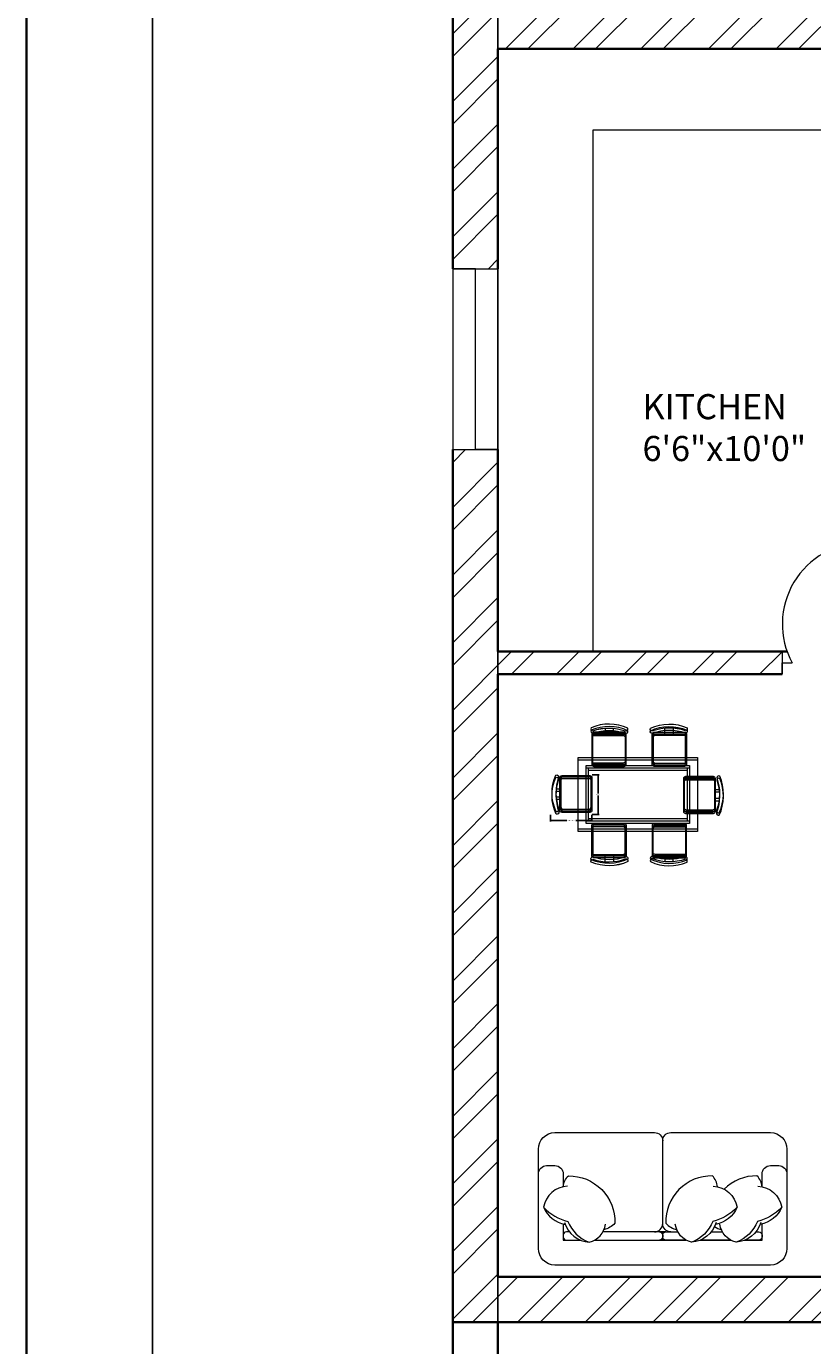
# Model space of a CAD drawing. Units: inches. Extents: x 2552 to 3217, y 1417 to 2737.
# Tile 2 of 25: x 2552 to 2709, y 1622 to 1885. Entities that reach past the tile are written whole.
import ezdxf

# ---------------------------------------------------------------- set-up
doc = ezdxf.new("R2010")
doc.units = ezdxf.units.IN
for name, color, linetype, lineweight in [('A-ANNO-DIMS', 2, 'Continuous', 18), ('A-ANNO-TTLB', 7, 'Continuous', 35), ('A-AREA-IDEN', 7, 'Continuous', 18), ('A-DOOR', 21, 'Continuous', 18), ('A-FLOR-CASE', 9, 'Continuous', 18), ('A-FURN', 8, 'Continuous', 13), ('A-GLAZ', 161, 'Continuous', 18), ('A-WALL', 7, 'Continuous', 35), ('A-WALL-PATT', 217, 'Continuous', 13)]:
    doc.layers.add(name, color=color, linetype=linetype, lineweight=lineweight)
doc.styles.get("Standard").update_dxf_attribs({"font": 'arial.ttf'})
doc.dimstyles.get("Standard").update_dxf_attribs({"dimtxt": 0.18, "dimasz": 0.18, "dimexe": 0.18, "dimexo": 0.0625, "dimgap": 0.09, "dimtad": 0, "dimtih": 1, "dimtoh": 1, "dimdec": 4, "dimzin": 0, "dimdsep": 46, "dimtxsty": 'Standard', "dimcen": 0.09, "dimadec": 0, "dimazin": 0, "dimtfac": 1, "dimtdec": 4, "dimtofl": 0, "dimtmove": 0, "dimatfit": 3, "dimfxl": 1, "dimtolj": 1, "dimtzin": 0, "dimarcsym": 0})

# ---------------------------------------------------------------- blocks, each defined once
blk = doc.blocks.new('TABLE-DINING-RECT')
for points in [[(0, 14.74), (23.77, 14.74), (23.77, 0.48), (0, 0.48)], [(0, 14.74), (23.77, 14.74), (23.77, 0.48), (0, 0.48)], [(0, 14.26), (23.77, 14.26), (23.77, 0), (0, 0)], [(0, 14.26), (23.77, 14.26), (23.77, 0), (0, 0)], [(1.58, 13.15), (22.19, 13.15), (22.19, 2.06), (1.58, 2.06)], [(1.58, 13.15), (22.19, 13.15), (22.19, 2.06), (1.58, 2.06)], [(1.58, 12.68), (22.19, 12.68), (22.19, 1.59), (1.58, 1.59)], [(1.58, 12.68), (22.19, 12.68), (22.19, 1.58), (1.58, 1.58)], [(2.06, 12.68), (21.71, 12.68), (21.71, 2.54), (2.06, 2.54)], [(2.06, 12.68), (21.71, 12.68), (21.71, 2.54), (2.06, 2.54)], [(2.06, 12.2), (21.71, 12.2), (21.71, 2.06), (2.06, 2.06)], [(2.06, 12.2), (21.71, 12.2), (21.71, 2.06), (2.06, 2.06)]]:
    blk.add_lwpolyline(points, close=True)
blk = doc.blocks.new('DINING-CHAIR-WEST')
for points in [[(1.37, 0.99, -0.578392), (0.83, 0.5, -0.214524), (0.73, 7.8, -0.552014), (1.32, 7.46, 0.175809), (1.37, 0.99)], [(1.37, 0.99, -0.578392), (0.83, 0.49, -0.214524), (0.73, 7.8, -0.552014), (1.32, 7.46, 0.175809), (1.37, 0.99)], [(1.37, 0.51, -0.578392), (0.83, 0.02, -0.214524), (0.73, 7.33, -0.552014), (1.32, 6.98, 0.175809), (1.37, 0.51)], [(1.37, 0.51, -0.578392), (0.83, 0.02, -0.214524), (0.73, 7.33, -0.552014), (1.32, 6.98, 0.175809), (1.37, 0.51)], [(1.58, 7.27, -0.414214), (2, 7.69), (7.53, 7.69, -0.414214), (7.95, 7.27), (7.95, 1.26, -0.414214), (7.53, 0.84), (2, 0.84, -0.414214), (1.58, 1.26), (1.58, 7.27)], [(1.58, 7.27, -0.414214), (2, 7.69), (7.53, 7.69, -0.414214), (7.95, 7.27), (7.95, 1.26, -0.414214), (7.53, 0.84), (2, 0.84, -0.414214), (1.58, 1.26), (1.58, 7.27)], [(1.58, 6.8, -0.414214), (2, 7.22), (7.53, 7.22, -0.414214), (7.95, 6.8), (7.95, 0.78, -0.414214), (7.53, 0.36), (2, 0.36, -0.414214), (1.58, 0.78), (1.58, 6.8)], [(1.58, 6.8, -0.414214), (2, 7.22), (7.53, 7.22, -0.414214), (7.95, 6.8), (7.95, 0.78, -0.414214), (7.53, 0.36), (2, 0.36, -0.414214), (1.58, 0.78), (1.58, 6.8)], [(1.58, 3.37), (0.82, 3.37, 0.064759)], [(1.58, 3.37), (0.82, 3.37, 0.064759)], [(1.58, 2.9), (0.82, 2.9, 0.064759)], [(1.58, 2.9), (0.82, 2.9, 0.064759)]]:
    blk.add_lwpolyline(points, format="xyb")
for points in [[(1.77, 7.27), (1.77, 1.45, 0.414214), (2.19, 1.03), (7.34, 1.03, 0.414214), (7.76, 1.45), (7.76, 7.27, 0.512069), (7.34, 7.5), (2.19, 7.5, 0.512069)], [(1.77, 7.27), (1.77, 1.45, 0.414214), (2.19, 1.03), (7.34, 1.03, 0.414214), (7.76, 1.45), (7.76, 7.27, 0.512069), (7.34, 7.5), (2.19, 7.5, 0.512069)], [(1.77, 6.79), (1.77, 0.97, 0.414214), (2.19, 0.55), (7.34, 0.55, 0.414214), (7.76, 0.97), (7.76, 6.79, 0.512069), (7.34, 7.03), (2.19, 7.03, 0.512069)], [(1.77, 6.79), (1.77, 0.97, 0.414214), (2.19, 0.55), (7.34, 0.55, 0.414214), (7.76, 0.97), (7.76, 6.79, 0.512069), (7.34, 7.03), (2.19, 7.03, 0.512069)]]:
    blk.add_lwpolyline(points, format="xyb", close=True)
for points in [[(0.81, 5.05), (1.58, 5.05)], [(0.81, 5.05), (1.58, 5.05)], [(0.81, 4.58), (1.58, 4.58)], [(0.81, 4.58), (1.58, 4.58)]]:
    blk.add_lwpolyline(points)
blk = doc.blocks.new('DINING-CHAIR-EAST')
for points in [[(6.37, 7.27, 0.414214), (5.95, 7.69), (0.42, 7.69, 0.414214), (0, 7.27), (0, 1.26, 0.414214), (0.42, 0.84), (5.95, 0.84, 0.414214), (6.37, 1.26), (6.37, 7.27)], [(6.37, 7.27, 0.414214), (5.95, 7.69), (0.42, 7.69, 0.414214), (0, 7.27), (0, 1.26, 0.414214), (0.42, 0.84), (5.95, 0.84, 0.414214), (6.37, 1.26), (6.37, 7.27)], [(6.37, 6.8, 0.414214), (5.95, 7.22), (0.42, 7.22, 0.414214), (0, 6.8), (0, 0.78, 0.414214), (0.42, 0.36), (5.95, 0.36, 0.414214), (6.37, 0.78), (6.37, 6.8)], [(6.37, 6.8, 0.414214), (5.95, 7.22), (0.42, 7.22, 0.414214), (0, 6.8), (0, 0.78, 0.414214), (0.42, 0.36), (5.95, 0.36, 0.414214), (6.37, 0.78), (6.37, 6.8)], [(6.63, 7.46, -0.175809), (6.58, 0.99, 0.578392), (7.12, 0.5, 0.214524), (7.22, 7.8, 0.552014), (6.63, 7.46, -0.065079)], [(6.63, 7.46, -0.175809), (6.58, 0.99, 0.578392), (7.12, 0.49, 0.214524), (7.22, 7.8, 0.552014), (6.63, 7.46, -0.065079)], [(6.63, 6.98, -0.175809), (6.58, 0.51, 0.578392), (7.12, 0.02, 0.214524), (7.22, 7.33, 0.552014), (6.63, 6.98, -0.065079)], [(6.63, 6.98, -0.175809), (6.58, 0.51, 0.578392), (7.12, 0.02, 0.214524), (7.22, 7.33, 0.552014), (6.63, 6.98, -0.065079)], [(6.37, 3.37), (7.13, 3.37, -0.064759)], [(6.37, 3.37), (7.13, 3.37, -0.064759)], [(6.37, 2.9), (7.13, 2.9, -0.064759)], [(6.37, 2.9), (7.13, 2.9, -0.064759)]]:
    blk.add_lwpolyline(points, format="xyb")
for points in [[(6.18, 7.27), (6.18, 1.45, -0.414214), (5.76, 1.03), (0.61, 1.03, -0.414214), (0.19, 1.45), (0.19, 7.27, -0.512069), (0.61, 7.5), (5.76, 7.5, -0.512069)], [(6.18, 7.27), (6.18, 1.45, -0.414214), (5.76, 1.03), (0.61, 1.03, -0.414214), (0.19, 1.45), (0.19, 7.27, -0.512069), (0.61, 7.5), (5.76, 7.5, -0.512069)], [(6.18, 6.79), (6.18, 0.97, -0.414214), (5.76, 0.55), (0.61, 0.55, -0.414214), (0.19, 0.97), (0.19, 6.79, -0.512069), (0.61, 7.03), (5.76, 7.03, -0.512069)], [(6.18, 6.79), (6.18, 0.97, -0.414214), (5.76, 0.55), (0.61, 0.55, -0.414214), (0.19, 0.97), (0.19, 6.79, -0.512069), (0.61, 7.03), (5.76, 7.03, -0.512069)]]:
    blk.add_lwpolyline(points, format="xyb", close=True)
for points in [[(7.14, 5.05), (6.37, 5.05)], [(7.14, 5.05), (6.37, 5.05)], [(7.14, 4.58), (6.37, 4.58)], [(7.14, 4.58), (6.37, 4.58)]]:
    blk.add_lwpolyline(points)
blk = doc.blocks.new('DINING-CHAIR-SOUTH-EAST')
for points in [[(6.8, 2.06, 0.414214), (7.22, 2.48), (7.22, 8.01, 0.414214), (6.8, 8.43), (0.78, 8.43, 0.414214), (0.36, 8.01), (0.36, 2.48, 0.414214), (0.78, 2.06), (6.8, 2.06)], [(6.8, 2.06, 0.414214), (7.22, 2.48), (7.22, 8.01, 0.414214), (6.8, 8.43), (0.78, 8.43, 0.414214), (0.36, 8.01), (0.36, 2.48, 0.414214), (0.78, 2.06), (6.8, 2.06)], [(6.8, 1.58, 0.414214), (7.22, 2), (7.22, 7.53, 0.414214), (6.8, 7.95), (0.78, 7.95, 0.414214), (0.36, 7.53), (0.36, 2, 0.414214), (0.78, 1.58), (6.8, 1.58)], [(6.8, 1.58, 0.414214), (7.22, 2), (7.22, 7.53, 0.414214), (6.8, 7.95), (0.78, 7.95, 0.414214), (0.36, 7.53), (0.36, 2, 0.414214), (0.78, 1.58), (6.8, 1.58)], [(6.98, 1.8, -0.175809), (0.51, 1.85, 0.578392), (0.02, 1.31, 0.214524), (7.33, 1.21, 0.552014), (6.98, 1.8, -0.065079)], [(6.98, 1.8, -0.175809), (0.51, 1.85, 0.578392), (0.02, 1.31, 0.214524), (7.33, 1.21, 0.552014), (6.98, 1.8, -0.065079)], [(6.98, 1.32, -0.175809), (0.51, 1.37, 0.578392), (0.02, 0.83, 0.214524), (7.33, 0.74, 0.552014), (6.98, 1.32, -0.065079)], [(6.98, 1.32, -0.175809), (0.51, 1.37, 0.578392), (0.02, 0.83, 0.214524), (7.33, 0.74, 0.552014), (6.98, 1.32, -0.065079)], [(2.9, 2.06), (2.9, 1.3, -0.064759)], [(2.9, 2.06), (2.9, 1.3, -0.064759)], [(2.9, 1.58), (2.9, 0.82, -0.064759)], [(2.9, 1.58), (2.9, 0.82, -0.064759)]]:
    blk.add_lwpolyline(points, format="xyb")
for points in [[(6.79, 2.25), (0.97, 2.25, -0.414214), (0.55, 2.67), (0.55, 7.82, -0.414214), (0.97, 8.24), (6.79, 8.24, -0.512069), (7.03, 7.82), (7.03, 2.67, -0.512069)], [(6.79, 2.25), (0.97, 2.25, -0.414214), (0.55, 2.67), (0.55, 7.82, -0.414214), (0.97, 8.24), (6.79, 8.24, -0.512069), (7.03, 7.82), (7.03, 2.67, -0.512069)], [(6.79, 1.77), (0.97, 1.77, -0.414214), (0.55, 2.19), (0.55, 7.34, -0.414214), (0.97, 7.76), (6.79, 7.76, -0.512069), (7.03, 7.34), (7.03, 2.19, -0.512069)], [(6.79, 1.77), (0.97, 1.77, -0.414214), (0.55, 2.19), (0.55, 7.34, -0.414214), (0.97, 7.76), (6.79, 7.76, -0.512069), (7.03, 7.34), (7.03, 2.19, -0.512069)]]:
    blk.add_lwpolyline(points, format="xyb", close=True)
for points in [[(4.58, 1.28), (4.58, 2.06)], [(4.58, 1.28), (4.58, 2.06)], [(4.58, 0.81), (4.58, 1.58)], [(4.58, 0.81), (4.58, 1.58)]]:
    blk.add_lwpolyline(points)
blk = doc.blocks.new('WIN-36')
for p, q in [((4.5, 36), (0, 36)), ((0, 36), (9, 36)), ((0, 36), (0, 0)), ((4.5, 0), (4.5, 36)), ((9, 36), (9, 0)), ((0, 0), (9, 0)), ((9, 0), (4.5, 0))]:
    blk.add_line(p, q)
blk = doc.blocks.new('*D37')
at = {"layer": 'A-ANNO-DIMS', "color": 0, "lineweight": -2, "transparency": 16777216}
for p, q in [((2656.84, 1727.55), (2656.84, 1726.2)), ((2657.02, 1726.38), (2660.07, 1726.38)), ((2664.89, 1726.38), (2661.83, 1726.38)), ((2665.07, 1727.55), (2665.07, 1726.2))]:
    blk.add_line(p, q, dxfattribs=at)
at = {"layer": 'A-ANNO-DIMS', "color": 0, "transparency": 16777216}
for points in [[(2657.02, 1726.41), (2657.02, 1726.35), (2656.84, 1726.38)], [(2664.89, 1726.41), (2664.89, 1726.35), (2665.07, 1726.38)]]:
    blk.add_solid(points, dxfattribs=at)
at = {"layer": 'Defpoints', "color": 0, "transparency": 16777216}
for p in [(2656.84, 1727.62), (2665.07, 1727.62), (2665.07, 1726.38)]:
    blk.add_point(p, dxfattribs=at)
at = {"layer": 'A-ANNO-DIMS', "color": 0, "transparency": 16777216, "insert": (2660.95, 1726.38), "char_height": 0.18, "attachment_point": 5}
blk.add_mtext('\\A1;CHAIR 8 TYP.', dxfattribs=at)
blk = doc.blocks.new('*D38')
at = {"layer": 'A-ANNO-DIMS', "color": 0, "lineweight": -2, "transparency": 16777216}
for p, q in [((2665.13, 1735.51), (2666.48, 1735.51)), ((2666.3, 1735.33), (2666.3, 1731.75)), ((2666.3, 1727.8), (2666.3, 1731.38)), ((2665.13, 1727.62), (2666.48, 1727.62))]:
    blk.add_line(p, q, dxfattribs=at)
at = {"layer": 'A-ANNO-DIMS', "color": 0, "transparency": 16777216}
for points in [[(2666.27, 1735.33), (2666.33, 1735.33), (2666.3, 1735.51)], [(2666.27, 1727.8), (2666.33, 1727.8), (2666.3, 1727.62)]]:
    blk.add_solid(points, dxfattribs=at)
at = {"layer": 'Defpoints', "color": 0, "transparency": 16777216}
for p in [(2665.07, 1735.51), (2666.3, 1735.51), (2665.07, 1727.62)]:
    blk.add_point(p, dxfattribs=at)
at = {"layer": 'A-ANNO-DIMS', "color": 0, "transparency": 16777216, "insert": (2666.3, 1731.56), "char_height": 0.18, "attachment_point": 5}
blk.add_mtext('\\A1;8 TYP.', dxfattribs=at)
blk = doc.blocks.new('*D50')
at = {"layer": 'A-ANNO-DIMS', "color": 0, "lineweight": -2, "transparency": 16777216}
for p, q in [((2637.29, 2649.51), (2577.37, 2649.51)), ((2577.55, 2649.33), (2577.55, 2096.19)), ((2577.55, 1542.69), (2577.55, 2095.83)), ((2637.29, 1542.51), (2577.37, 1542.51))]:
    blk.add_line(p, q, dxfattribs=at)
at = {"layer": 'A-ANNO-DIMS', "color": 0, "transparency": 16777216}
for points in [[(2577.52, 2649.33), (2577.58, 2649.33), (2577.55, 2649.51)], [(2577.52, 1542.69), (2577.58, 1542.69), (2577.55, 1542.51)]]:
    blk.add_solid(points, dxfattribs=at)
at = {"layer": 'Defpoints', "color": 0, "transparency": 16777216}
for p in [(2577.55, 2649.51), (2637.35, 2649.51), (2637.35, 1542.51)]:
    blk.add_point(p, dxfattribs=at)
at = {"layer": 'A-ANNO-DIMS', "color": 0, "transparency": 16777216, "insert": (2577.55, 2096.01), "char_height": 0.18, "attachment_point": 5}
blk.add_mtext('\\A1;1107', dxfattribs=at)
blk = doc.blocks.new('*D64')
at = {"layer": 'A-ANNO-DIMS', "color": 0, "lineweight": -2, "transparency": 16777216}
for p, q in [((2646.35, 1551.58), (2646.35, 2709.49)), ((2646.53, 2709.31), (2802.77, 2709.31)), ((2959.93, 2709.31), (2803.69, 2709.31)), ((2960.11, 1551.58), (2960.11, 2709.49))]:
    blk.add_line(p, q, dxfattribs=at)
at = {"layer": 'A-ANNO-DIMS', "color": 0, "transparency": 16777216}
for points in [[(2646.53, 2709.34), (2646.53, 2709.28), (2646.35, 2709.31)], [(2959.93, 2709.34), (2959.93, 2709.28), (2960.11, 2709.31)]]:
    blk.add_solid(points, dxfattribs=at)
at = {"layer": 'Defpoints', "color": 0, "transparency": 16777216}
for p in [(2960.11, 2709.31), (2646.35, 1551.51), (2960.11, 1551.51)]:
    blk.add_point(p, dxfattribs=at)
at = {"layer": 'A-ANNO-DIMS', "color": 0, "transparency": 16777216, "insert": (2803.23, 2709.31), "char_height": 0.18, "attachment_point": 5}
blk.add_mtext('\\A1;313.76', dxfattribs=at)

msp = doc.modelspace()

# ---------------------------------------------------------------- hatches: boundary and pattern name
at = {"layer": 'A-WALL-PATT'}
h = msp.add_hatch(dxfattribs=at)
h.set_pattern_fill('ANSI32', color=256)
h.paths.add_polyline_path([(2756.676, 2649.5125), (2637.3535, 2649.5125), (2637.3535, 2617.9626), (2641.8535, 2617.9626), (2646.3535, 2617.9626), (2646.3535, 2640.5125), (2724.3535, 2640.5125), (2724.3535, 2520.5125), (2720.299, 2520.5125), (2720.299, 2516.0125), (2733.4075, 2516.0125), (2733.4075, 2518.2213), (2733.4075, 2520.5125), (2728.8535, 2520.5125), (2728.8535, 2640.5125), (2756.676, 2640.5125)])
h.paths.add_polyline_path([(2848.8535, 2649.5125), (2804.676, 2649.5125), (2804.676, 2640.5125), (2839.8535, 2640.5125), (2839.8535, 2598.3517), (2848.8535, 2598.3517)])
h.paths.add_polyline_path([(2646.3535, 2516.0125), (2697.9593, 2516.0125), (2697.9593, 2518.2625), (2697.9593, 2520.5125), (2646.3535, 2520.5125), (2646.3535, 2581.9626), (2637.3535, 2581.9626), (2637.3535, 2364.3298), (2646.3535, 2364.3298), (2646.3535, 2387.0125), (2724.3535, 2387.0125), (2724.3535, 2267.0125), (2721.0443, 2267.0125), (2721.0443, 2262.5125), (2733.7854, 2262.5125), (2733.7854, 2264.7625), (2733.7854, 2267.0125), (2728.8535, 2267.0125), (2728.8535, 2387.0125), (2839.8535, 2387.0125), (2839.8535, 2363.8387), (2848.8535, 2363.8387), (2848.8535, 2403.7415), (2844.3535, 2403.7415), (2839.8535, 2403.7415), (2839.8535, 2396.0125), (2646.3535, 2396.0125)])
h.paths.add_polyline_path([(2848.8535, 2550.3517), (2844.3535, 2550.3517), (2839.8535, 2550.3517), (2839.8535, 2520.5125), (2801.9195, 2520.5125), (2801.9195, 2518.2625), (2801.9195, 2516.0125), (2839.8535, 2516.0125), (2839.8535, 2507.5813), (2848.8535, 2507.5813)], flags=17)
h.paths.add_polyline_path([(2848.8535, 2483.5813), (2844.3535, 2483.5813), (2839.8535, 2483.5813), (2839.8535, 2468.0125), (2773.8535, 2468.0125), (2773.8535, 2516.0125), (2778.1336, 2516.0125), (2778.1336, 2520.5125), (2766.696, 2520.5125), (2766.696, 2518.2625), (2766.696, 2516.0125), (2769.3535, 2516.0125), (2769.3535, 2463.5125), (2839.8535, 2463.5125), (2839.8535, 2431.0782), (2848.8535, 2431.0782)], flags=17)
h.paths.add_polyline_path([(2917.8535, 2569.2764), (2913.3535, 2569.2764), (2908.8535, 2569.2764), (2908.8535, 2433.001), (2917.8535, 2433.001), (2917.8535, 2516.0125), (2967.486, 2516.0125), (2967.486, 2520.5125), (2917.8535, 2520.5125)])
h.paths.add_polyline_path([(3000.3535, 2640.5125), (2995.8535, 2640.5125), (2995.8535, 2520.5125), (2990.688, 2520.5125), (2990.688, 2516.0125), (3004.0844, 2516.0125), (3004.0844, 2518.2625), (3004.0844, 2520.5125), (3000.3535, 2520.5125)])
h.paths.add_polyline_path([(3120.3535, 2561.3689), (3115.8535, 2561.3689), (3111.3535, 2561.3689), (3111.3535, 2520.5125), (3070.9814, 2520.5125), (3070.9814, 2518.2625), (3070.9814, 2516.0125), (3111.3535, 2516.0125), (3111.3535, 2505.1841), (3120.3535, 2505.1841)])
h.paths.add_polyline_path([(3120.3535, 2481.1841), (3115.8535, 2481.1841), (3111.3535, 2481.1841), (3111.3535, 2468.0125), (3045.3535, 2468.0125), (3045.3535, 2516.0125), (3048.9787, 2516.0125), (3048.9787, 2520.5125), (3036.3395, 2520.5125), (3036.3395, 2516.0125), (3040.8535, 2516.0125), (3040.8535, 2463.5125), (3111.3535, 2463.5125), (3111.3535, 2396.0125), (2917.8535, 2396.0125), (2917.8535, 2403.4124), (2913.3535, 2403.4124), (2908.8535, 2403.4124), (2908.8535, 2182.5756), (2917.8535, 2182.5756), (2917.8535, 2262.5125), (2968.001, 2262.5125), (2968.001, 2264.7625), (2968.001, 2267.0125), (2917.8535, 2267.0125), (2917.8535, 2387.0125), (3111.3535, 2387.0125), (3111.3535, 2352.2435), (3120.3535, 2352.2435)])
h.paths.add_polyline_path([(3120.3535, 2304.2435), (3115.8535, 2304.2435), (3111.3535, 2304.2435), (3111.3535, 2267.0125), (3073.8616, 2267.0125), (3073.8616, 2264.7625), (3073.8616, 2262.5125), (3111.3535, 2262.5125), (3111.3535, 2252.376), (3120.3535, 2252.376)], flags=17)
h.paths.add_polyline_path([(3120.3535, 2228.376), (3115.8535, 2228.376), (3111.3535, 2228.376), (3111.3535, 2214.5125), (3045.3535, 2214.5125), (3045.3535, 2262.5125), (3049.3096, 2262.5125), (3049.3096, 2267.0125), (3035.0125, 2267.0125), (3035.0125, 2262.5125), (3040.8535, 2262.5125), (3040.8535, 2210.0125), (3111.3535, 2210.0125), (3111.3535, 2142.5125), (2917.8535, 2142.5125), (2917.8535, 2150.2408), (2913.3535, 2150.2408), (2908.8535, 2150.2408), (2908.8535, 1924.9905), (2917.8535, 1924.9905), (2917.8535, 2009.0125), (2971.959, 2009.0125), (2971.959, 2011.2625), (2971.959, 2013.5125), (2917.8535, 2013.5125), (2917.8535, 2133.5125), (2995.8535, 2133.5125), (2995.8535, 2013.5125), (2992.1797, 2013.5125), (2992.1797, 2009.0125), (3004.3344, 2009.0125), (3004.3344, 2011.2625), (3004.3344, 2013.5125), (3000.3535, 2013.5125), (3000.3535, 2133.5125), (3111.3535, 2133.5125), (3111.3535, 2115.0291), (3120.3535, 2115.0291)])
h.paths.add_polyline_path([(3000.3535, 2387.0125), (2995.8535, 2387.0125), (2995.8535, 2267.0125), (2991.3326, 2267.0125), (2991.3326, 2262.5125), (3004.1044, 2262.5125), (3004.1044, 2264.7625), (3004.1044, 2267.0125), (3000.3535, 2267.0125)], flags=17)
h.paths.add_polyline_path([(3120.3535, 1973.2388), (3115.8535, 1973.2388), (3111.3535, 1973.2388), (3111.3535, 1961.0125), (3045.3535, 1961.0125), (3045.3535, 2009.0125), (3048.9101, 2009.0125), (3048.9101, 2013.5125), (3037.105, 2013.5125), (3037.105, 2011.2625), (3037.105, 2009.0125), (3040.8535, 2009.0125), (3040.8535, 1956.5125), (3111.3535, 1956.5125), (3111.3535, 1889.0125), (2917.8535, 1889.0125), (2917.8535, 1895.7215), (2913.3535, 1895.7215), (2908.8535, 1895.7215), (2908.8535, 1844.2217), (2917.8535, 1844.2217), (2917.8535, 1880.0125), (3111.3535, 1880.0125), (3111.3535, 1846.9541), (3120.3535, 1846.9541)])
h.paths.add_polyline_path([(3120.3535, 2067.0291), (3111.3535, 2067.0291), (3111.3535, 2013.5125), (3071.3001, 2013.5125), (3071.3001, 2009.0125), (3111.3535, 2009.0125), (3111.3535, 1997.2388), (3120.3535, 1997.2388)], flags=0)
h.paths.add_polyline_path([(3120.3535, 1798.9541), (3115.8535, 1798.9541), (3111.3535, 1798.9541), (3111.3535, 1760.0125), (3071.2497, 1760.0125), (3071.2497, 1757.7625), (3071.2497, 1755.5125), (3111.3535, 1755.5125), (3111.3535, 1746.162), (3120.3535, 1746.2478)])
h.paths.add_polyline_path([(3120.3535, 1722.2049), (3111.3535, 1722.2049), (3111.3535, 1707.5125), (3045.3535, 1707.5125), (3045.3535, 1755.5125), (3048.6624, 1755.5125), (3048.6624, 1760.0125), (3035.3703, 1760.0125), (3035.3703, 1755.5125), (3040.8535, 1755.5125), (3040.8535, 1703.0125), (3111.3535, 1703.0125), (3111.3535, 1635.5125), (2917.8535, 1635.5125), (2917.8535, 1643.1366), (2913.3535, 1643.1366), (2908.8535, 1643.1366), (2908.8535, 1626.5125), (3120.3535, 1626.5125)])
h.paths.add_polyline_path([(2917.8535, 1755.5125), (2973.2287, 1755.5125), (2973.2287, 1757.7625), (2973.2287, 1760.0125), (2917.8535, 1760.0125), (2917.8535, 1808.2217), (2913.3535, 1808.2217), (2908.8535, 1808.2217), (2908.8535, 1676.1665), (2917.8535, 1676.1665)])
h.paths.add_polyline_path([(3000.3535, 1880.0125), (2995.8535, 1880.0125), (2995.8535, 1760.0125), (2992.9329, 1760.0125), (2992.9329, 1755.5125), (3003.8766, 1755.5125), (3003.8766, 1757.7625), (3003.8766, 1760.0125), (3000.3535, 1760.0125)])
h.paths.add_polyline_path([(2848.8535, 1896.6971), (2844.3535, 1896.6971), (2839.8535, 1896.6971), (2839.8535, 1889.0125), (2646.3535, 1889.0125), (2646.3535, 2009.0125), (2700.5253, 2009.0125), (2700.5253, 2011.2625), (2700.5253, 2013.5125), (2646.3535, 2013.5125), (2646.3535, 2053.1812), (2641.8535, 2053.1812), (2637.3535, 2053.1812), (2637.3535, 1836.254), (2646.3535, 1836.254), (2646.3535, 1880.0125), (2724.3535, 1880.0125), (2724.3535, 1760.0125), (2721.2473, 1760.0125), (2721.2473, 1755.5125), (2731.9187, 1755.5125), (2731.9187, 1757.7625), (2731.9187, 1760.0125), (2728.8535, 1760.0125), (2728.8535, 1880.0125), (2839.8535, 1880.0125), (2839.8535, 1840.3813), (2848.8535, 1840.3813)])
h.paths.add_polyline_path([(2848.8535, 1792.3813), (2844.3535, 1792.3813), (2839.8535, 1792.3813), (2839.8535, 1760.0125), (2797.8845, 1760.0125), (2797.8845, 1755.5125), (2839.8535, 1755.5125), (2839.8535, 1743.3688), (2844.3535, 1743.3688), (2848.8535, 1743.3688)], flags=0)
h.paths.add_polyline_path([(2848.8535, 1719.3688), (2844.3535, 1719.3688), (2839.8535, 1719.3688), (2839.8535, 1707.5125), (2773.8535, 1707.5125), (2773.8535, 1755.5125), (2777.716, 1755.5125), (2777.716, 1760.0125), (2760.9247, 1760.0125), (2760.9247, 1757.9721), (2760.9247, 1755.5125), (2769.3535, 1755.5125), (2769.3535, 1703.0125), (2839.8535, 1703.0125), (2839.8535, 1673.0277), (2848.8535, 1672.9407)], flags=0)
h.paths.add_polyline_path([(2646.3535, 1755.5125), (2702.9171, 1755.5125), (2702.9171, 1757.7625), (2702.9171, 1760.0125), (2646.3535, 1760.0125), (2646.3535, 1800.254), (2641.8535, 1800.254), (2637.3535, 1800.254), (2637.3535, 1626.5125), (2848.8535, 1626.5125), (2848.8535, 1643.1187), (2844.3535, 1643.1187), (2839.8535, 1643.1187), (2839.8535, 1635.5125), (2646.3535, 1635.5125)])
h.paths.add_polyline_path([(2848.8535, 2148.8427), (2844.3535, 2148.8427), (2839.8535, 2148.8427), (2839.8535, 2142.5125), (2646.3535, 2142.5125), (2646.3535, 2262.5125), (2701.3562, 2262.5125), (2701.3562, 2264.7625), (2701.3562, 2267.0125), (2646.3535, 2267.0125), (2646.3535, 2328.3298), (2637.3535, 2328.3298), (2637.3535, 2089.1812), (2646.3535, 2089.1812), (2646.3535, 2133.5125), (2839.8535, 2133.5125), (2839.8535, 2097.5966), (2848.8535, 2097.5966)])
h.paths.add_polyline_path([(2728.8535, 2133.5125), (2724.3535, 2133.5125), (2724.3535, 2013.5125), (2719.6039, 2013.5125), (2719.6039, 2009.0125), (2732.5784, 2009.0125), (2732.5784, 2011.2625), (2732.5784, 2013.5125), (2728.8535, 2013.5125)])
h.paths.add_polyline_path([(2848.8535, 1970.0557), (2844.3535, 1970.0557), (2839.8535, 1970.0557), (2839.8535, 1961.0125), (2773.8535, 1961.0125), (2773.8535, 2009.0125), (2777.3388, 2009.0125), (2777.3388, 2013.5125), (2764.7681, 2013.5125), (2764.7681, 2009.0125), (2769.3535, 2009.0125), (2769.3535, 1956.5125), (2839.8535, 1956.5125), (2839.8535, 1924.7199), (2848.8535, 1924.7199)], flags=17)
h.paths.add_polyline_path([(2848.8535, 2049.5966), (2844.3535, 2049.5966), (2839.8535, 2049.5966), (2839.8535, 2013.5125), (2798.198, 2013.5125), (2798.198, 2011.2625), (2798.198, 2009.0125), (2839.8535, 2009.0125), (2839.8535, 1994.0557), (2848.8535, 1994.0557)], flags=17)
h.paths.add_polyline_path([(2848.8535, 2315.8387), (2839.8535, 2315.8387), (2839.8535, 2267.0125), (2799.3375, 2267.0125), (2799.3375, 2264.7625), (2799.3375, 2262.5125), (2839.8535, 2262.5125), (2839.8535, 2253.2843), (2848.8535, 2253.2843)], flags=17)
h.paths.add_polyline_path([(2848.8535, 2229.2843), (2839.8535, 2229.2843), (2839.8535, 2177.6936), (2848.8535, 2177.6936)], flags=17)
h.paths.add_polyline_path([(2839.8535, 2214.5125), (2773.8535, 2214.5125), (2773.8535, 2262.5125), (2777.6984, 2262.5125), (2777.6984, 2267.0125), (2763.8226, 2267.0125), (2763.8226, 2262.5125), (2769.3535, 2262.5125), (2769.3535, 2210.0125), (2839.8535, 2210.0125)], flags=17)
h.paths.add_polyline_path([(3050.32, 2520.2817), (3088.9114, 2520.2817), (3088.9114, 2538.939), (3050.32, 2538.939)], flags=9)

# ---------------------------------------------------------------- linework, layer by layer
at = {"layer": 'A-ANNO-TTLB'}
msp.add_lwpolyline([(2552.473, 2736.5692), (3216.7862, 2736.5692), (3216.7862, 1416.6914), (2552.473, 1416.6914)], close=True, dxfattribs=at)
at = {"layer": 'A-DOOR'}
for p, q in [((2702.9171, 1760.0125), (2702.9171, 1755.5125)), ((2702.9171, 1755.5125), (2702.9171, 1757.7625)), ((2702.9171, 1757.7625), (2704.9171, 1757.7625))]:
    msp.add_line(p, q, dxfattribs=at)
msp.add_arc((2719.2473, 1765.4843), 16.2782, 90, 208.31787, dxfattribs=at)
at = {"layer": 'A-FLOR-CASE'}
for p, q in [((2665.3321, 1760.0125), (2665.3321, 1863.9064)), ((2665.3321, 1863.9064), (2724.3535, 1863.9064))]:
    msp.add_line(p, q, dxfattribs=at)
at = {"layer": 'A-FURN'}
for points in [[(2665.2615, 1744.2633, -0.17580919), (2671.7359, 1744.2143, 0.57839206), (2672.2264, 1744.7536, 0.21452438), (2664.9181, 1744.8517, 0.55201397), (2665.2615, 1744.2633, -0.06507904)], [(2665.2615, 1743.7879, -0.17580919), (2671.7359, 1743.7389, 0.57839206), (2672.2264, 1744.2782, 0.21452438), (2664.9181, 1744.3763, 0.55201397), (2665.2615, 1743.7879, -0.06507904)], [(2665.2615, 1744.2631, -0.17580919), (2671.7359, 1744.2141, 0.57839206), (2672.2264, 1744.7534, 0.21452438), (2664.9181, 1744.8515, 0.55201397), (2665.2615, 1744.2631, -0.06507904)], [(2665.2615, 1743.7877, -0.17580919), (2671.7359, 1743.7387, 0.57839206), (2672.2264, 1744.278, 0.21452438), (2664.9181, 1744.376, 0.55201397), (2665.2615, 1743.7877, -0.06507904)], [(2669.35, 1744.0035), (2669.35, 1744.7637, -0.06475861)], [(2669.35, 1744.0032), (2669.35, 1744.7634, -0.06475861)], [(2669.35, 1743.5281), (2669.35, 1744.2882, -0.06475861)], [(2669.35, 1743.5278), (2669.35, 1744.288, -0.06475861)], [(2677.1866, 1744.2143, -0.57839206), (2676.6961, 1744.7536, -0.21452438), (2684.0044, 1744.8517, -0.55201397), (2683.661, 1744.2633, 0.1758092), (2677.1866, 1744.2143)], [(2677.1866, 1744.2141, -0.57839206), (2676.6961, 1744.7534, -0.21452438), (2684.0044, 1744.8515, -0.55201397), (2683.661, 1744.2631, 0.1758092), (2677.1866, 1744.2141)], [(2677.1866, 1743.7389, -0.57839206), (2676.6961, 1744.2782, -0.21452438), (2684.0044, 1744.3763, -0.55201397), (2683.661, 1743.7879, 0.1758092), (2677.1866, 1743.7389)], [(2677.1866, 1743.7387, -0.57839206), (2676.6961, 1744.278, -0.21452438), (2684.0044, 1744.376, -0.55201397), (2683.661, 1743.7877, 0.1758092), (2677.1866, 1743.7387)], [(2679.5725, 1744.0035), (2679.5725, 1744.7637, 0.06475861)], [(2679.5725, 1744.0032), (2679.5725, 1744.7634, 0.06475861)], [(2679.5725, 1743.5281), (2679.5725, 1744.2882, 0.06475861)], [(2679.5725, 1743.5278), (2679.5725, 1744.288, 0.06475861)], [(2671.4612, 1744.0035), (2665.4506, 1744.0035, 0.41421356), (2665.0301, 1743.583), (2665.0301, 1738.0563, 0.41421356), (2665.4506, 1737.6358), (2671.4612, 1737.6358, 0.41421356), (2671.8818, 1738.0563), (2671.8818, 1743.583, 0.41421356), (2671.4612, 1744.0035)], [(2671.4613, 1744.0032), (2665.4506, 1744.0032, 0.41421356), (2665.0301, 1743.5827), (2665.0301, 1738.056, 0.41421356), (2665.4506, 1737.6355), (2671.4613, 1737.6355, 0.41421356), (2671.8818, 1738.056), (2671.8818, 1743.5827, 0.41421356), (2671.4613, 1744.0032)], [(2671.4612, 1743.5281), (2665.4506, 1743.5281, 0.41421356), (2665.0301, 1743.1076), (2665.0301, 1737.5809, 0.41421356), (2665.4506, 1737.1604), (2671.4612, 1737.1604, 0.41421356), (2671.8818, 1737.5809), (2671.8818, 1743.1076, 0.41421356), (2671.4612, 1743.5281)], [(2671.4613, 1743.5278), (2665.4506, 1743.5278, 0.41421356), (2665.0301, 1743.1073), (2665.0301, 1737.5806, 0.41421356), (2665.4506, 1737.1601), (2671.4613, 1737.1601, 0.41421356), (2671.8818, 1737.5806), (2671.8818, 1743.1073, 0.41421356), (2671.4613, 1743.5278)], [(2683.4719, 1744.0035, -0.41421356), (2683.8924, 1743.583), (2683.8924, 1738.0563, -0.41421356), (2683.4719, 1737.6358), (2677.4613, 1737.6358, -0.41421356), (2677.0408, 1738.0563), (2677.0408, 1743.583, -0.41421356), (2677.4613, 1744.0035), (2683.4719, 1744.0035)], [(2683.4719, 1744.0032, -0.41421356), (2683.8925, 1743.5827), (2683.8925, 1738.056, -0.41421356), (2683.4719, 1737.6355), (2677.4613, 1737.6355, -0.41421356), (2677.0408, 1738.056), (2677.0408, 1743.5827, -0.41421356), (2677.4613, 1744.0032), (2683.4719, 1744.0032)], [(2683.4719, 1743.5281, -0.41421356), (2683.8924, 1743.1076), (2683.8924, 1737.5809, -0.41421356), (2683.4719, 1737.1604), (2677.4613, 1737.1604, -0.41421356), (2677.0408, 1737.5809), (2677.0408, 1743.1076, -0.41421356), (2677.4613, 1743.5281), (2683.4719, 1743.5281)], [(2683.4719, 1743.5278, -0.41421356), (2683.8925, 1743.1073), (2683.8925, 1737.5806, -0.41421356), (2683.4719, 1737.1601), (2677.4613, 1737.1601, -0.41421356), (2677.0408, 1737.5806), (2677.0408, 1743.1073, -0.41421356), (2677.4613, 1743.5278), (2683.4719, 1743.5278)], [(2671.4612, 1719.436), (2665.4506, 1719.436, -0.41421356), (2665.0301, 1719.8565), (2665.0301, 1725.3832, -0.41421356), (2665.4506, 1725.8037), (2671.4612, 1725.8037, -0.41421356), (2671.8818, 1725.3832), (2671.8818, 1719.8565, -0.41421356), (2671.4612, 1719.436)], [(2671.4613, 1719.4358), (2665.4506, 1719.4358, -0.41421356), (2665.0301, 1719.8563), (2665.0301, 1725.383, -0.41421356), (2665.4506, 1725.8035), (2671.4613, 1725.8035, -0.41421356), (2671.8818, 1725.383), (2671.8818, 1719.8563, -0.41421356), (2671.4613, 1719.4358)], [(2671.4612, 1718.9606), (2665.4506, 1718.9606, -0.41421356), (2665.0301, 1719.3811), (2665.0301, 1724.9078, -0.41421356), (2665.4506, 1725.3283), (2671.4612, 1725.3283, -0.41421356), (2671.8818, 1724.9078), (2671.8818, 1719.3811, -0.41421356), (2671.4612, 1718.9606)], [(2671.4613, 1718.9603), (2665.4506, 1718.9603, -0.41421356), (2665.0301, 1719.3809), (2665.0301, 1724.9076, -0.41421356), (2665.4506, 1725.3281), (2671.4613, 1725.3281, -0.41421356), (2671.8818, 1724.9076), (2671.8818, 1719.3809, -0.41421356), (2671.4613, 1718.9603)], [(2671.7359, 1719.2252, -0.57839206), (2672.2264, 1718.6859, -0.21452438), (2664.9181, 1718.5878, -0.55201397), (2665.2615, 1719.1762, 0.17580929), (2671.7359, 1719.2252)], [(2671.7359, 1718.7498, -0.57839206), (2672.2264, 1718.2104, -0.21452438), (2664.9181, 1718.1124, -0.55201397), (2665.2615, 1718.7007, 0.17580929), (2671.7359, 1718.7498)], [(2671.7359, 1719.2249, -0.57839206), (2672.2264, 1718.6856, -0.21452438), (2664.9181, 1718.5875, -0.55201397), (2665.2615, 1719.1759, 0.17580929), (2671.7359, 1719.2249)], [(2671.7359, 1718.7495, -0.57839206), (2672.2264, 1718.2102, -0.21452438), (2664.9181, 1718.1121, -0.55201397), (2665.2615, 1718.7005, 0.17580929), (2671.7359, 1718.7495)], [(2669.35, 1719.436), (2669.35, 1718.6758, 0.06475861)], [(2669.35, 1719.4358), (2669.35, 1718.6756, 0.06475861)], [(2669.35, 1718.9606), (2669.35, 1718.2004, 0.06475861)], [(2669.35, 1718.9603), (2669.35, 1718.2002, 0.06475861)], [(2677.494, 1644.4721, 0.41421356), (2679.1436, 1646.1217), (2679.1436, 1662.6173, 0.41421356)], [(2680.7932, 1644.4721, -0.41421356), (2679.1436, 1646.1217), (2679.1436, 1662.6173, -0.41421356)], [(2654.4001, 1656.0191, -0.41421356), (2656.0497, 1657.6686), (2657.6993, 1657.6686, -0.41421356), (2659.3488, 1656.0191), (2659.3488, 1653.4633)], [(2698.9384, 1653.4633), (2698.9384, 1656.0191, -0.41421356), (2700.5879, 1657.6686), (2702.2375, 1657.6686, -0.41421356), (2703.887, 1656.0191)], [(2659.3452, 1653.4625, -0.16554063), (2660.3657, 1655.6421, -0.42598917), (2669.63, 1646.1923, -0.12152332), (2667.4308, 1644.8898, 7.11546429)], [(2690.0558, 1653.4625, 0.16554063), (2689.0353, 1655.6421, 0.42598917), (2679.7711, 1646.1923, 0.12152332), (2681.9702, 1644.8898, -7.11546429)], [(2698.9419, 1653.4625, 0.16554063), (2697.9215, 1655.6421, 0.20023115), (2691.3733, 1652.9876, 0.12152332)], [(2660.1767, 1653.5631, 0.35677236), (2655.45, 1649.4052, 0.24954205), (2659.7328, 1645.9787, -9.61688035)], [(2689.2244, 1653.5631, -0.35677236), (2693.9511, 1649.4052, -0.24954205), (2689.6683, 1645.9787, 9.61688035)], [(2698.1105, 1653.5631, -0.35677236), (2702.8372, 1649.4052, -0.24954205), (2698.5544, 1645.9787, 9.61688035)], [(2655.45, 1649.4052, 0.14772988), (2660.2712, 1646.5703, 0.21334276), (2664.5252, 1642.4123, 0.17866181)], [(2693.9511, 1649.4052, -0.14772988), (2689.1299, 1646.5703, -0.21334276), (2684.8759, 1642.4123, -0.17866181)], [(2702.8372, 1649.4052, -0.14772988), (2698.016, 1646.5703, -0.21334276), (2693.762, 1642.4123, -0.17866181)], [(2660.6076, 1644.4721), (2660.0087, 1644.4721, 0.41421356), (2659.3488, 1643.8123), (2659.3488, 1643.4824, 0.41421356), (2660.0087, 1642.8225)], [(2659.6051, 1646.3443, 0.30666349), (2664.5252, 1642.4123, 0.30632997), (2667.7393, 1646.0033, -0.87284716)], [(2665.5633, 1642.8225), (2678.4838, 1642.8225, 0.41421356), (2679.1436, 1643.4824), (2679.1436, 1643.8123, 0.41421356), (2678.4838, 1644.4721), (2667.2243, 1644.4721, 0.41421356)], [(2677.494, 1644.4721, 0.41421356), (2679.1436, 1646.1217)], [(2680.7932, 1644.4721, -0.41421356), (2679.1436, 1646.1217)], [(2683.8377, 1642.8225), (2679.8034, 1642.8225, -0.41421356), (2679.1436, 1643.4824), (2679.1436, 1643.8123, -0.41421356), (2679.8034, 1644.4721), (2682.1767, 1644.4721, -0.41421356)], [(2689.7959, 1646.3443, -0.30666349), (2684.8759, 1642.4123, -0.30632997), (2681.6617, 1646.0033, 0.87284716)], [(2688.7934, 1644.4721), (2691.0628, 1644.4721, -0.41421356)], [(2689.4734, 1645.5347, 0.07186538), (2690.8564, 1644.8898, -7.11546429)], [(2698.6821, 1646.3443, -0.30666349), (2693.762, 1642.4123, -0.30632997), (2690.5479, 1646.0033, 0.87284716)], [(2695.4681, 1642.8225), (2698.9384, 1642.8225), (2698.9384, 1646.0643, -0.41421356)], [(2697.6795, 1644.4721), (2698.2785, 1644.4721, -0.41421356), (2698.9384, 1643.8123), (2698.9384, 1643.4824, -0.41421356), (2698.2785, 1642.8225)], [(2660.0087, 1642.8225), (2662.8191, 1642.8225, 0.41421356)], [(2692.7239, 1642.8225), (2686.582, 1642.8225, -0.41421356)], [(2698.2785, 1642.8225), (2695.4681, 1642.8225, -0.41421356)]]:
    msp.add_lwpolyline(points, format="xyb", dxfattribs=at)
for points in [[(2667.6675, 1744.7775), (2667.6675, 1744.0035)], [(2667.6675, 1744.7772), (2667.6675, 1744.0032)], [(2667.6675, 1744.3021), (2667.6675, 1743.5281)], [(2667.6675, 1744.3018), (2667.6675, 1743.5278)], [(2681.255, 1744.7775), (2681.255, 1744.0035)], [(2681.255, 1744.7772), (2681.255, 1744.0032)], [(2681.255, 1744.3021), (2681.255, 1743.5281)], [(2681.255, 1744.3018), (2681.255, 1743.5278)], [(2667.6675, 1718.662), (2667.6675, 1719.436)], [(2667.6675, 1718.6618), (2667.6675, 1719.4358)], [(2667.6675, 1718.1866), (2667.6675, 1718.9606)], [(2667.6675, 1718.1864), (2667.6675, 1718.9603)], [(2659.3488, 1646.0643), (2659.3488, 1642.8225), (2662.8191, 1642.8225)], [(2665.5633, 1642.8225), (2683.8377, 1642.8225)], [(2686.582, 1642.8225), (2692.7239, 1642.8225)]]:
    msp.add_lwpolyline(points, dxfattribs=at)
for points in [[(2665.4531, 1743.814), (2671.2718, 1743.814, -0.41421356), (2671.6923, 1743.3935), (2671.6923, 1738.2457, -0.41421356), (2671.2718, 1737.8252), (2665.4531, 1737.8252, -0.51206948), (2665.2195, 1738.2457), (2665.2195, 1743.3935, -0.51206948)], [(2665.4531, 1743.8138), (2671.2718, 1743.8138, -0.41421356), (2671.6923, 1743.3933), (2671.6923, 1738.2455, -0.41421356), (2671.2718, 1737.825), (2665.4531, 1737.825, -0.51206948), (2665.2195, 1738.2455), (2665.2195, 1743.3933, -0.51206948)], [(2665.4531, 1743.3386), (2671.2718, 1743.3386, -0.41421356), (2671.6923, 1742.9181), (2671.6923, 1737.7703, -0.41421356), (2671.2718, 1737.3498), (2665.4531, 1737.3498, -0.51206948), (2665.2195, 1737.7703), (2665.2195, 1742.9181, -0.51206948)], [(2665.4531, 1743.3384), (2671.2718, 1743.3384, -0.41421356), (2671.6923, 1742.9179), (2671.6923, 1737.7701, -0.41421356), (2671.2718, 1737.3496), (2665.4531, 1737.3496, -0.51206948), (2665.2195, 1737.7701), (2665.2195, 1742.9179, -0.51206948)], [(2683.4694, 1743.814), (2677.6507, 1743.814, 0.41421356), (2677.2302, 1743.3935), (2677.2302, 1738.2457, 0.41421356), (2677.6507, 1737.8252), (2683.4694, 1737.8252, 0.51206948), (2683.703, 1738.2457), (2683.703, 1743.3935, 0.51206948)], [(2683.4694, 1743.8138), (2677.6507, 1743.8138, 0.41421356), (2677.2302, 1743.3933), (2677.2302, 1738.2455, 0.41421356), (2677.6507, 1737.825), (2683.4694, 1737.825, 0.51206948), (2683.703, 1738.2455), (2683.703, 1743.3933, 0.51206948)], [(2683.4694, 1743.3386), (2677.6507, 1743.3386, 0.41421356), (2677.2302, 1742.9181), (2677.2302, 1737.7703, 0.41421356), (2677.6507, 1737.3498), (2683.4694, 1737.3498, 0.51206948), (2683.703, 1737.7703), (2683.703, 1742.9181, 0.51206948)], [(2683.4694, 1743.3384), (2677.6507, 1743.3384, 0.41421356), (2677.2302, 1742.9179), (2677.2302, 1737.7701, 0.41421356), (2677.6507, 1737.3496), (2683.4694, 1737.3496, 0.51206948), (2683.703, 1737.7701), (2683.703, 1742.9179, 0.51206948)], [(2665.4531, 1719.6255), (2671.2718, 1719.6255, 0.41421356), (2671.6923, 1720.046), (2671.6923, 1725.1938, 0.41421356), (2671.2718, 1725.6143), (2665.4531, 1725.6143, 0.51206948), (2665.2195, 1725.1938), (2665.2195, 1720.046, 0.51206948)], [(2665.4531, 1719.6252), (2671.2718, 1719.6252, 0.41421356), (2671.6923, 1720.0457), (2671.6923, 1725.1935, 0.41421356), (2671.2718, 1725.614), (2665.4531, 1725.614, 0.51206948), (2665.2195, 1725.1935), (2665.2195, 1720.0457, 0.51206948)], [(2665.4531, 1719.15), (2671.2718, 1719.15, 0.41421356), (2671.6923, 1719.5706), (2671.6923, 1724.7184, 0.41421356), (2671.2718, 1725.1389), (2665.4531, 1725.1389, 0.51206948), (2665.2195, 1724.7184), (2665.2195, 1719.5706, 0.51206948)], [(2665.4531, 1719.1498), (2671.2718, 1719.1498, 0.41421356), (2671.6923, 1719.5703), (2671.6923, 1724.7181, 0.41421356), (2671.2718, 1725.1386), (2665.4531, 1725.1386, 0.51206948), (2665.2195, 1724.7181), (2665.2195, 1719.5703, 0.51206948)], [(2678.4838, 1642.8225), (2679.8034, 1642.8225, -0.41421356), (2679.1436, 1643.4824), (2679.1436, 1643.8123, -0.41421356), (2679.8034, 1644.4721), (2678.4838, 1644.4721, -0.41421356), (2679.1436, 1643.8123), (2679.1436, 1643.4824, -0.41421356)]]:
    msp.add_lwpolyline(points, format="xyb", close=True, dxfattribs=at)
at = {"layer": 'A-FURN', "ltscale": 0.03}
msp.add_lwpolyline([(2677.494, 1664.2669, -0.41421356), (2679.1436, 1662.6173, -0.41421356), (2680.7932, 1664.2669), (2700.5879, 1664.2669, -0.41421356), (2703.887, 1660.9677), (2703.887, 1641.173, -0.41421356), (2700.5879, 1637.8739), (2657.6993, 1637.8739, -0.41421356), (2654.4001, 1641.173), (2654.4001, 1660.9677, -0.41421356), (2657.6993, 1664.2669), (2677.494, 1664.2669, -0.41421356), (2679.1436, 1662.6173, -0.41421356), (2680.7932, 1664.2669)], format="xyb", dxfattribs=at)
at = {"layer": 'A-GLAZ'}
msp.add_line((2646.3535, 1800.254), (2646.3535, 1800.254), dxfattribs=at)
at = {"layer": 'A-WALL'}
for p, q in [((2637.3535, 2053.1812), (2637.3535, 1836.254)), ((2646.3535, 1880.0125), (2724.3535, 1880.0125)), ((2646.3535, 1880.0125), (2646.3535, 1836.254)), ((2637.3535, 1800.254), (2637.3535, 1626.5125)), ((2646.3535, 1800.254), (2646.3535, 1760.0125)), ((2646.3535, 1760.0125), (2703.9163, 1760.0125)), ((2646.3535, 1755.5125), (2702.9171, 1755.5125)), ((2646.3535, 1755.5125), (2646.3535, 1635.5125)), ((2646.3535, 1635.5125), (2839.8535, 1635.5125)), ((2637.3535, 1626.5125), (2848.8535, 1626.5125)), ((2637.3535, 1542.5125), (2637.3535, 1626.5125)), ((2646.3535, 1551.5125), (2646.3535, 1626.5125))]:
    msp.add_line(p, q, dxfattribs=at)

# ---------------------------------------------------------------- block references
at = {"layer": 'A-FURN'}
for name, p in [('TABLE-DINING-RECT', (2662.3217, 1724.1891)), ('DINING-CHAIR-WEST', (2657.1157, 1727.6429)), ('DINING-CHAIR-EAST', (2683.283, 1727.437)), ('DINING-CHAIR-SOUTH-EAST', (2676.6767, 1717.3771))]:
    msp.add_blockref(name, p, dxfattribs=at)
at = {"layer": 'A-GLAZ'}
msp.add_blockref('WIN-36', (2637.354, 1800.2543), dxfattribs=at)

# ---------------------------------------------------------------- texts
at = {"layer": 'A-AREA-IDEN', "insert": (2675.1246, 1811.2928), "char_height": 5, "attachment_point": 1}
msp.add_mtext_dynamic_manual_height_columns('KITCHEN\\P6\'6"x10\'0"', width=136.352736, gutter_width=12.5, heights=[0], dxfattribs=at)

# ---------------------------------------------------------------- dimensions: what is measured, and where the dimension line sits
at = {"layer": 'A-ANNO-DIMS'}
dim = msp.add_linear_dim(base=(2960.1089, 2709.3125), p1=(2646.3535, 1551.5125), p2=(2960.1089, 1551.5125), dimstyle='Standard', override={"dimdec": 2, "dimlfac": 1, "dimrnd": 0, "dimzin": 0, "dimdsep": 46, "dimlunit": 2}, dxfattribs=at)
dim.commit()
dim.dimension.update_dxf_attribs({"geometry": '*D64', "text_midpoint": (2803.2312, 2709.3125)})
dim = msp.add_linear_dim(base=(2577.5535, 2649.5125), p1=(2637.3535, 1542.5125), p2=(2637.3535, 2649.5125), angle=90, dimstyle='Standard', override={"dimdec": 0, "dimlfac": 1, "dimrnd": 0, "dimzin": 0, "dimdsep": 46, "dimlunit": 2}, dxfattribs=at)
dim.commit()
dim.dimension.update_dxf_attribs({"geometry": '*D50', "text_midpoint": (2577.5535, 2096.0125)})
dim = msp.add_linear_dim(base=(2666.301, 1735.5103), p1=(2665.0665, 1727.6164), p2=(2665.0665, 1735.5103), angle=90, text='<> TYP.', dimstyle='Standard', override={"dimdec": 0, "dimlfac": 1, "dimrnd": 0, "dimzin": 0, "dimdsep": 46, "dimlunit": 2}, dxfattribs=at)
dim.commit()
dim.dimension.update_dxf_attribs({"geometry": '*D38', "text_midpoint": (2666.301, 1731.5633)})
dim = msp.add_linear_dim(base=(2665.0665, 1726.3819), p1=(2656.8365, 1727.6164), p2=(2665.0665, 1727.6164), text='CHAIR <> TYP.', dimstyle='Standard', override={"dimdec": 0, "dimlfac": 1, "dimrnd": 0, "dimzin": 0, "dimdsep": 46, "dimlunit": 2}, dxfattribs=at)
dim.commit()
dim.dimension.update_dxf_attribs({"geometry": '*D37', "text_midpoint": (2660.9515, 1726.3819)})

doc.saveas('drawing.dxf')
